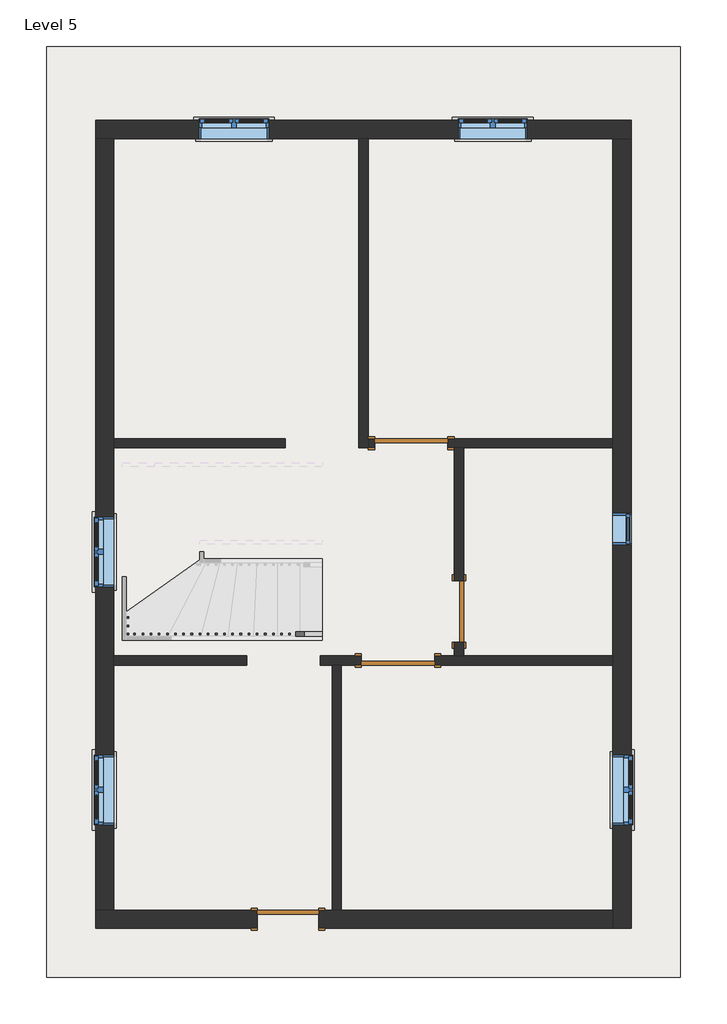
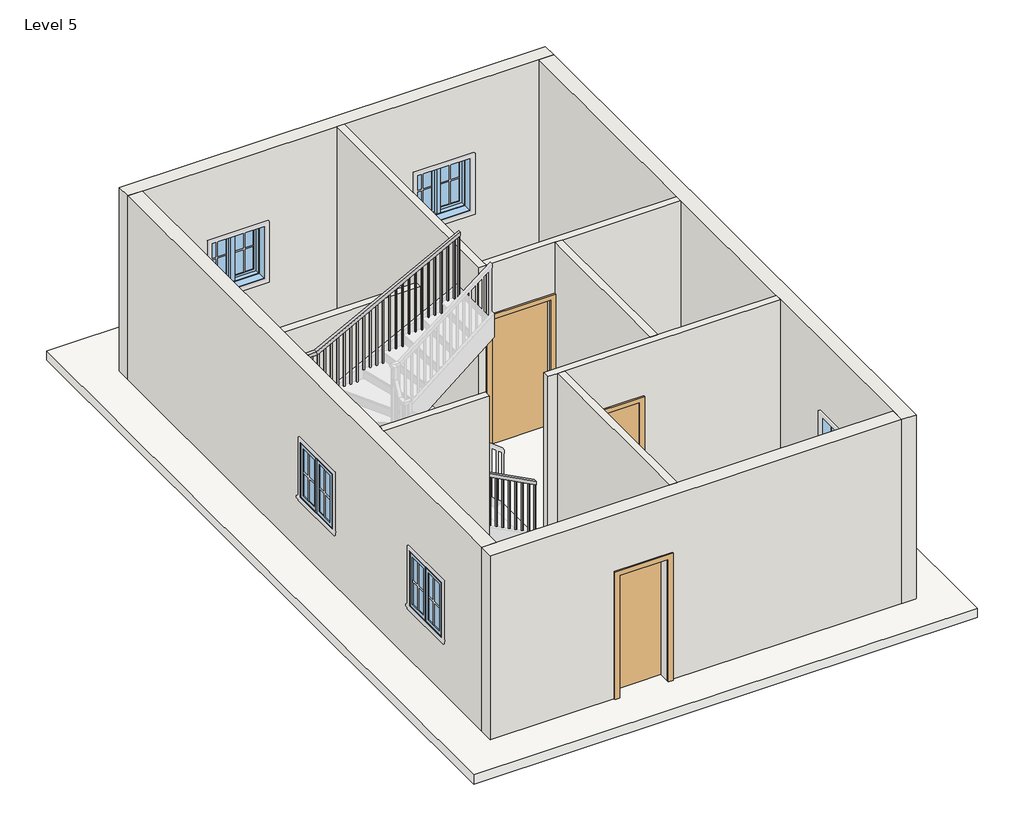
# One storey, part 1 of 2: 11 walls, 6 windows, 4 doors, 1 railing, 1 roof.
"""IFC4 building model written with IfcOpenShell, lengths in millimetres."""

from ifc_helpers import new_model, si_unit, frame, origin, place, context, project, spatial, polyline, outline, extrude, faceted_brep, transform, mapped, element, save
from components import door_d8f5dbb5, door_85036156, door_305aa2a5, door_e5f9f3c4, window_aa618e30, window_339605e1

model = new_model("IFC4")

# Units and contexts
model_context = context("Model", 3, world=origin())
ifc_project = project(units=[si_unit("LENGTHUNIT", "METRE", prefix="MILLI")], contexts=[model_context])

# Site, building, storey
site = spatial("IfcSite", under=ifc_project)
building = spatial("IfcBuilding", under=site)
storey = spatial("IfcBuildingStorey", under=building, Name="Level 5", Elevation=9601.2)

# Doors
placement = place(None, origin())
door_shape = door_d8f5dbb5(model_context)
element("IfcDoor", 1, ObjectType="Single-Flush : 30\" x 80\"", at=placement, inside=storey, context=model_context, shape_type="MappedRepresentation", body=[
    mapped(door_shape, transform((-82.2715692, -955.3070853, 9601.2), x_axis=(0.0, -1.0, 0.0), y_axis=(1.0, 0.0, 0.0), z_axis=(0.0, 0.0, 1.0))),
])
door_2_shape = door_85036156(model_context)
element("IfcDoor", 2, ObjectType="Single-Flush : 30\" x 80\"", at=placement, inside=storey, context=model_context, shape_type="MappedRepresentation", body=[
    mapped(door_2_shape, transform((-2212.5949167, -4784.3570853, 9601.2), x_axis=(-1.0, 0.0, 0.0), y_axis=(0.0, -1.0, 0.0), z_axis=(0.0, 0.0, 1.0))),
])
door_3_shape = door_305aa2a5(model_context)
element("IfcDoor", 3, ObjectType="Single-Flush : 36\" x 84\"", at=placement, inside=storey, context=model_context, shape_type="MappedRepresentation", body=[
    mapped(door_3_shape, transform((-677.5332429, 1140.1929147, 9601.2), x_axis=(-1.0, 0.0, 0.0), y_axis=(0.0, -1.0, 0.0), z_axis=(0.0, 0.0, 1.0))),
])
door_4_shape = door_e5f9f3c4(model_context)
element("IfcDoor", 4, ObjectType="Single-Flush : 36\" x 84\"", at=placement, inside=storey, context=model_context, shape_type="MappedRepresentation", body=[
    mapped(door_4_shape, transform((-842.6332429, -1564.9070853, 9601.2), x_axis=(-1.0, 0.0, 0.0), y_axis=(0.0, -1.0, 0.0), z_axis=(0.0, 0.0, 1.0))),
])

# Railing
element("IfcRailing", 5, ObjectType="Handrail - Rectangular", at=placement, inside=storey, context=model_context, shape_type="SolidModel", body=[
    faceted_brep([(-1783.4132248, -1260.1070853, 10684.9333333), (-1783.4132248, -1260.1070853, 10627.4742652), (-1783.4132248, -1209.3070853, 10627.4742652), (-1783.4132248, -1209.3070853, 10684.9333333), (-4041.1382869, -1260.1070853, 11878.2239201), (-4053.7373514, -1260.1070853, 11827.4239201), (-4053.7373514, -1209.3070853, 11827.4239201), (-4041.1382869, -1209.3070853, 11878.2239201), (-4225.5449167, -1260.1070853, 11878.2239201), (-4225.5449167, -1260.1070853, 11827.4239201), (-4174.7449167, -1209.3070853, 11827.4239201), (-4174.7449167, -1209.3070853, 11878.2239201), (-4225.5449167, -972.7952032, 11878.2239201), (-4225.5449167, -964.8446271, 11827.4239201), (-4174.7449167, -964.8446271, 11827.4239201), (-4174.7449167, -972.7952032, 11878.2239201), (-4225.5449167, 560.7810325, 12370.3094132), (-4225.5449167, 568.7316087, 12319.5094132), (-4174.7449167, 568.7316087, 12319.5094132), (-4174.7449167, 560.7810325, 12370.3094132), (-4225.5449167, 848.0929147, 12370.3094132), (-4225.5449167, 848.0929147, 12319.5094132), (-4174.7449167, 797.2929147, 12319.5094132), (-4174.7449167, 797.2929147, 12370.3094132), (-4041.1382869, 848.0929147, 12370.3094132), (-4028.5392223, 848.0929147, 12319.5094132), (-4028.5392223, 797.2929147, 12319.5094132), (-4041.1382869, 797.2929147, 12370.3094132), (-1783.4132248, 848.0929147, 13563.6), (-1783.4132248, 797.2929147, 13563.6), (-1783.4132248, 797.2929147, 13506.1409318), (-1783.4132248, 848.0929147, 13506.1409318)], [[[0, 1, 2, 3]], [[1, 0, 4, 5]], [[2, 1, 5, 6]], [[3, 2, 6, 7]], [[0, 3, 7, 4]], [[5, 4, 8, 9]], [[6, 5, 9, 10]], [[7, 6, 10, 11]], [[4, 7, 11, 8]], [[9, 8, 12, 13]], [[10, 9, 13, 14]], [[11, 10, 14, 15]], [[8, 11, 15, 12]], [[13, 12, 16, 17]], [[14, 13, 17, 18]], [[15, 14, 18, 19]], [[12, 15, 19, 16]], [[17, 16, 20, 21]], [[18, 17, 21, 22]], [[19, 18, 22, 23]], [[16, 19, 23, 20]], [[21, 20, 24, 25]], [[22, 21, 25, 26]], [[23, 22, 26, 27]], [[20, 23, 27, 24]], [[28, 29, 30, 31]], [[25, 24, 28, 31]], [[26, 25, 31, 30]], [[27, 26, 30, 29]], [[24, 27, 29, 28]]]),
    extrude(outline(polyline([(13458.8597858, -1872.8699167), (12479.8666667, -1872.8699167), (12479.8666667, -1853.8199167), (13468.9284102, -1853.8199167), (13458.8597858, -1872.8699167)])), frame((0.0, 813.1679147, 0.0), z_axis=(0.0, 1.0, 0.0), x_axis=(0.0, 0.0, 1.0)), (0.0, 0.0, 1.0), 19.05),
    extrude(outline(polyline([(13405.1604556, -1974.4699167), (12479.8666667, -1974.4699167), (12479.8666667, -1955.4199167), (13415.22908, -1955.4199167), (13405.1604556, -1974.4699167)])), frame((0.0, 813.1679147, 0.0), z_axis=(0.0, 1.0, 0.0), x_axis=(0.0, 0.0, 1.0)), (0.0, 0.0, 1.0), 19.05),
    extrude(outline(polyline([(13351.4611254, -2076.0699167), (12310.5333333, -2076.0699167), (12310.5333333, -2057.0199167), (13361.5297498, -2057.0199167), (13351.4611254, -2076.0699167)])), frame((0.0, 813.1679147, 0.0), z_axis=(0.0, 1.0, 0.0), x_axis=(0.0, 0.0, 1.0)), (0.0, 0.0, 1.0), 19.05),
    extrude(outline(polyline([(13297.7617952, -2177.6699167), (12310.5333333, -2177.6699167), (12310.5333333, -2158.6199167), (13307.8304196, -2158.6199167), (13297.7617952, -2177.6699167)])), frame((0.0, 813.1679147, 0.0), z_axis=(0.0, 1.0, 0.0), x_axis=(0.0, 0.0, 1.0)), (0.0, 0.0, 1.0), 19.05),
    extrude(outline(polyline([(13244.062465, -2279.2699167), (12310.5333333, -2279.2699167), (12310.5333333, -2260.2199167), (13254.1310894, -2260.2199167), (13244.062465, -2279.2699167)])), frame((0.0, 813.1679147, 0.0), z_axis=(0.0, 1.0, 0.0), x_axis=(0.0, 0.0, 1.0)), (0.0, 0.0, 1.0), 19.05),
    extrude(outline(polyline([(13190.3631348, -2380.8699167), (12141.2, -2380.8699167), (12141.2, -2361.8199167), (13200.4317592, -2361.8199167), (13190.3631348, -2380.8699167)])), frame((0.0, 813.1679147, 0.0), z_axis=(0.0, 1.0, 0.0), x_axis=(0.0, 0.0, 1.0)), (0.0, 0.0, 1.0), 19.05),
    extrude(outline(polyline([(13136.6638046, -2482.4699167), (12141.2, -2482.4699167), (12141.2, -2463.4199167), (13146.732429, -2463.4199167), (13136.6638046, -2482.4699167)])), frame((0.0, 813.1679147, 0.0), z_axis=(0.0, 1.0, 0.0), x_axis=(0.0, 0.0, 1.0)), (0.0, 0.0, 1.0), 19.05),
    extrude(outline(polyline([(13082.9644744, -2584.0699167), (12141.2, -2584.0699167), (12141.2, -2565.0199167), (13093.0330988, -2565.0199167), (13082.9644744, -2584.0699167)])), frame((0.0, 813.1679147, 0.0), z_axis=(0.0, 1.0, 0.0), x_axis=(0.0, 0.0, 1.0)), (0.0, 0.0, 1.0), 19.05),
    extrude(outline(polyline([(13029.2651442, -2685.6699167), (11971.8666667, -2685.6699167), (11971.8666667, -2666.6199167), (13039.3337686, -2666.6199167), (13029.2651442, -2685.6699167)])), frame((0.0, 813.1679147, 0.0), z_axis=(0.0, 1.0, 0.0), x_axis=(0.0, 0.0, 1.0)), (0.0, 0.0, 1.0), 19.05),
    extrude(outline(polyline([(12975.565814, -2787.2699167), (11971.8666667, -2787.2699167), (11971.8666667, -2768.2199167), (12985.6344384, -2768.2199167), (12975.565814, -2787.2699167)])), frame((0.0, 813.1679147, 0.0), z_axis=(0.0, 1.0, 0.0), x_axis=(0.0, 0.0, 1.0)), (0.0, 0.0, 1.0), 19.05),
    extrude(outline(polyline([(12921.8664838, -2888.8699167), (11971.8666667, -2888.8699167), (11971.8666667, -2869.8199167), (12931.9351082, -2869.8199167), (12921.8664838, -2888.8699167)])), frame((0.0, 813.1679147, 0.0), z_axis=(0.0, 1.0, 0.0), x_axis=(0.0, 0.0, 1.0)), (0.0, 0.0, 1.0), 19.05),
    extrude(outline(polyline([(12868.1671536, -2990.4699167), (11802.5333333, -2990.4699167), (11802.5333333, -2971.4199167), (12878.235778, -2971.4199167), (12868.1671536, -2990.4699167)])), frame((0.0, 813.1679147, 0.0), z_axis=(0.0, 1.0, 0.0), x_axis=(0.0, 0.0, 1.0)), (0.0, 0.0, 1.0), 19.05),
    extrude(outline(polyline([(12814.4678234, -3092.0699167), (11802.5333333, -3092.0699167), (11802.5333333, -3073.0199167), (12824.5364478, -3073.0199167), (12814.4678234, -3092.0699167)])), frame((0.0, 813.1679147, 0.0), z_axis=(0.0, 1.0, 0.0), x_axis=(0.0, 0.0, 1.0)), (0.0, 0.0, 1.0), 19.05),
    extrude(outline(polyline([(12760.7684932, -3193.6699167), (11802.5333333, -3193.6699167), (11802.5333333, -3174.6199167), (12770.8371176, -3174.6199167), (12760.7684932, -3193.6699167)])), frame((0.0, 813.1679147, 0.0), z_axis=(0.0, 1.0, 0.0), x_axis=(0.0, 0.0, 1.0)), (0.0, 0.0, 1.0), 19.05),
    extrude(outline(polyline([(12707.069163, -3295.2699167), (11802.5333333, -3295.2699167), (11802.5333333, -3276.2199167), (12717.1377874, -3276.2199167), (12707.069163, -3295.2699167)])), frame((0.0, 813.1679147, 0.0), z_axis=(0.0, 1.0, 0.0), x_axis=(0.0, 0.0, 1.0)), (0.0, 0.0, 1.0), 19.05),
    extrude(outline(polyline([(12653.3698328, -3396.8699167), (11633.2, -3396.8699167), (11633.2, -3377.8199167), (12663.4384572, -3377.8199167), (12653.3698328, -3396.8699167)])), frame((0.0, 813.1679147, 0.0), z_axis=(0.0, 1.0, 0.0), x_axis=(0.0, 0.0, 1.0)), (0.0, 0.0, 1.0), 19.05),
    extrude(outline(polyline([(12599.6705026, -3498.4699167), (11633.2, -3498.4699167), (11633.2, -3479.4199167), (12609.739127, -3479.4199167), (12599.6705026, -3498.4699167)])), frame((0.0, 813.1679147, 0.0), z_axis=(0.0, 1.0, 0.0), x_axis=(0.0, 0.0, 1.0)), (0.0, 0.0, 1.0), 19.05),
    extrude(outline(polyline([(12545.9711724, -3600.0699167), (11633.2, -3600.0699167), (11633.2, -3581.0199167), (12556.0397968, -3581.0199167), (12545.9711724, -3600.0699167)])), frame((0.0, 813.1679147, 0.0), z_axis=(0.0, 1.0, 0.0), x_axis=(0.0, 0.0, 1.0)), (0.0, 0.0, 1.0), 19.05),
    extrude(outline(polyline([(12492.2718422, -3701.6699167), (11633.2, -3701.6699167), (11633.2, -3682.6199167), (12502.3404666, -3682.6199167), (12492.2718422, -3701.6699167)])), frame((0.0, 813.1679147, 0.0), z_axis=(0.0, 1.0, 0.0), x_axis=(0.0, 0.0, 1.0)), (0.0, 0.0, 1.0), 19.05),
    extrude(outline(polyline([(12438.572512, -3803.2699167), (11463.8666667, -3803.2699167), (11463.8666667, -3784.2199167), (12448.6411364, -3784.2199167), (12438.572512, -3803.2699167)])), frame((0.0, 813.1679147, 0.0), z_axis=(0.0, 1.0, 0.0), x_axis=(0.0, 0.0, 1.0)), (0.0, 0.0, 1.0), 19.05),
    extrude(outline(polyline([(12384.8731818, -3904.8699167), (11463.8666667, -3904.8699167), (11463.8666667, -3885.8199167), (12394.9418062, -3885.8199167), (12384.8731818, -3904.8699167)])), frame((0.0, 813.1679147, 0.0), z_axis=(0.0, 1.0, 0.0), x_axis=(0.0, 0.0, 1.0)), (0.0, 0.0, 1.0), 19.05),
    extrude(outline(polyline([(12331.1738516, -4006.4699167), (11463.8666667, -4006.4699167), (11463.8666667, -3987.4199167), (12341.242476, -3987.4199167), (12331.1738516, -4006.4699167)])), frame((0.0, 813.1679147, 0.0), z_axis=(0.0, 1.0, 0.0), x_axis=(0.0, 0.0, 1.0)), (0.0, 0.0, 1.0), 19.05),
    extrude(outline(polyline([(-4108.0699167, 832.2179147), (-4089.0199167, 832.2179147), (-4089.0199167, 813.1679147), (-4108.0699167, 813.1679147), (-4108.0699167, 832.2179147)])), frame((0.0, 0.0, 11463.8666667), z_axis=(0.0, 0.0, 1.0), x_axis=(1.0, 0.0, 0.0)), (0.0, 0.0, 1.0), 855.6427466),
    extrude(outline(polyline([(-4209.6699167, 787.7679147), (-4209.6699167, 806.8179147), (-4190.6199167, 806.8179147), (-4190.6199167, 787.7679147), (-4209.6699167, 787.7679147)])), frame((0.0, 0.0, 11463.8666667), z_axis=(0.0, 0.0, 1.0), x_axis=(1.0, 0.0, 0.0)), (0.0, 0.0, 1.0), 855.6427466),
    extrude(outline(polyline([(-4209.6699167, 686.1679147), (-4209.6699167, 705.2179147), (-4190.6199167, 705.2179147), (-4190.6199167, 686.1679147), (-4209.6699167, 686.1679147)])), frame((0.0, 0.0, 11463.8666667), z_axis=(0.0, 0.0, 1.0), x_axis=(1.0, 0.0, 0.0)), (0.0, 0.0, 1.0), 855.6427466),
    extrude(outline(polyline([(-4209.6699167, 584.5679147), (-4209.6699167, 603.6179147), (-4190.6199167, 603.6179147), (-4190.6199167, 584.5679147), (-4209.6699167, 584.5679147)])), frame((0.0, 0.0, 11463.8666667), z_axis=(0.0, 0.0, 1.0), x_axis=(1.0, 0.0, 0.0)), (0.0, 0.0, 1.0), 855.6427466),
    extrude(outline(polyline([(502.0179147, 12298.1026907), (502.0179147, 11294.5333333), (482.9679147, 11294.5333333), (482.9679147, 12291.9900316), (502.0179147, 12298.1026907)])), frame((-4209.6699167, 0.0, 0.0), z_axis=(1.0, 0.0, 0.0), x_axis=(0.0, 1.0, 0.0)), (0.0, 0.0, 1.0), 19.05),
    extrude(outline(polyline([(400.4179147, 12265.5018425), (400.4179147, 11294.5333333), (381.3679147, 11294.5333333), (381.3679147, 12259.3891834), (400.4179147, 12265.5018425)])), frame((-4209.6699167, 0.0, 0.0), z_axis=(1.0, 0.0, 0.0), x_axis=(0.0, 1.0, 0.0)), (0.0, 0.0, 1.0), 19.05),
    extrude(outline(polyline([(298.8179147, 12232.9009942), (298.8179147, 11294.5333333), (279.7679147, 11294.5333333), (279.7679147, 12226.7883352), (298.8179147, 12232.9009942)])), frame((-4209.6699167, 0.0, 0.0), z_axis=(1.0, 0.0, 0.0), x_axis=(0.0, 1.0, 0.0)), (0.0, 0.0, 1.0), 19.05),
    extrude(outline(polyline([(197.2179147, 12200.300146), (197.2179147, 11294.5333333), (178.1679147, 11294.5333333), (178.1679147, 12194.187487), (197.2179147, 12200.300146)])), frame((-4209.6699167, 0.0, 0.0), z_axis=(1.0, 0.0, 0.0), x_axis=(0.0, 1.0, 0.0)), (0.0, 0.0, 1.0), 19.05),
    extrude(outline(polyline([(95.6179147, 12167.6992978), (95.6179147, 11294.5333333), (76.5679147, 11294.5333333), (76.5679147, 12161.5866387), (95.6179147, 12167.6992978)])), frame((-4209.6699167, 0.0, 0.0), z_axis=(1.0, 0.0, 0.0), x_axis=(0.0, 1.0, 0.0)), (0.0, 0.0, 1.0), 19.05),
    extrude(outline(polyline([(-5.9820853, 12135.0984495), (-5.9820853, 11125.2), (-25.0320853, 11125.2), (-25.0320853, 12128.9857905), (-5.9820853, 12135.0984495)])), frame((-4209.6699167, 0.0, 0.0), z_axis=(1.0, 0.0, 0.0), x_axis=(0.0, 1.0, 0.0)), (0.0, 0.0, 1.0), 19.05),
    extrude(outline(polyline([(-107.5820853, 12102.4976013), (-107.5820853, 11125.2), (-126.6320853, 11125.2), (-126.6320853, 12096.3849423), (-107.5820853, 12102.4976013)])), frame((-4209.6699167, 0.0, 0.0), z_axis=(1.0, 0.0, 0.0), x_axis=(0.0, 1.0, 0.0)), (0.0, 0.0, 1.0), 19.05),
    extrude(outline(polyline([(-209.1820853, 12069.8967531), (-209.1820853, 11125.2), (-228.2320853, 11125.2), (-228.2320853, 12063.784094), (-209.1820853, 12069.8967531)])), frame((-4209.6699167, 0.0, 0.0), z_axis=(1.0, 0.0, 0.0), x_axis=(0.0, 1.0, 0.0)), (0.0, 0.0, 1.0), 19.05),
    extrude(outline(polyline([(-310.7820853, 12037.2959049), (-310.7820853, 11125.2), (-329.8320853, 11125.2), (-329.8320853, 12031.1832458), (-310.7820853, 12037.2959049)])), frame((-4209.6699167, 0.0, 0.0), z_axis=(1.0, 0.0, 0.0), x_axis=(0.0, 1.0, 0.0)), (0.0, 0.0, 1.0), 19.05),
    extrude(outline(polyline([(-412.3820853, 12004.6950566), (-412.3820853, 11125.2), (-431.4320853, 11125.2), (-431.4320853, 11998.5823976), (-412.3820853, 12004.6950566)])), frame((-4209.6699167, 0.0, 0.0), z_axis=(1.0, 0.0, 0.0), x_axis=(0.0, 1.0, 0.0)), (0.0, 0.0, 1.0), 19.05),
    extrude(outline(polyline([(-513.9820853, 11972.0942084), (-513.9820853, 10955.8666667), (-533.0320853, 10955.8666667), (-533.0320853, 11965.9815494), (-513.9820853, 11972.0942084)])), frame((-4209.6699167, 0.0, 0.0), z_axis=(1.0, 0.0, 0.0), x_axis=(0.0, 1.0, 0.0)), (0.0, 0.0, 1.0), 19.05),
    extrude(outline(polyline([(-615.5820853, 11939.4933602), (-615.5820853, 10955.8666667), (-634.6320853, 10955.8666667), (-634.6320853, 11933.3807011), (-615.5820853, 11939.4933602)])), frame((-4209.6699167, 0.0, 0.0), z_axis=(1.0, 0.0, 0.0), x_axis=(0.0, 1.0, 0.0)), (0.0, 0.0, 1.0), 19.05),
    extrude(outline(polyline([(-717.1820853, 11906.892512), (-717.1820853, 10955.8666667), (-736.2320853, 10955.8666667), (-736.2320853, 11900.7798529), (-717.1820853, 11906.892512)])), frame((-4209.6699167, 0.0, 0.0), z_axis=(1.0, 0.0, 0.0), x_axis=(0.0, 1.0, 0.0)), (0.0, 0.0, 1.0), 19.05),
    extrude(outline(polyline([(-818.7820853, 11874.2916637), (-818.7820853, 10955.8666667), (-837.8320853, 10955.8666667), (-837.8320853, 11868.1790047), (-818.7820853, 11874.2916637)])), frame((-4209.6699167, 0.0, 0.0), z_axis=(1.0, 0.0, 0.0), x_axis=(0.0, 1.0, 0.0)), (0.0, 0.0, 1.0), 19.05),
    extrude(outline(polyline([(-920.3820853, 11841.6908155), (-920.3820853, 10955.8666667), (-939.4320853, 10955.8666667), (-939.4320853, 11835.5781565), (-920.3820853, 11841.6908155)])), frame((-4209.6699167, 0.0, 0.0), z_axis=(1.0, 0.0, 0.0), x_axis=(0.0, 1.0, 0.0)), (0.0, 0.0, 1.0), 19.05),
    extrude(outline(polyline([(-4209.6699167, -1041.0320853), (-4209.6699167, -1021.9820853), (-4190.6199167, -1021.9820853), (-4190.6199167, -1041.0320853), (-4209.6699167, -1041.0320853)])), frame((0.0, 0.0, 10786.5333333), z_axis=(0.0, 0.0, 1.0), x_axis=(1.0, 0.0, 0.0)), (0.0, 0.0, 1.0), 1040.8905868),
    extrude(outline(polyline([(-4209.6699167, -1142.6320853), (-4209.6699167, -1123.5820853), (-4190.6199167, -1123.5820853), (-4190.6199167, -1142.6320853), (-4209.6699167, -1142.6320853)])), frame((0.0, 0.0, 10786.5333333), z_axis=(0.0, 0.0, 1.0), x_axis=(1.0, 0.0, 0.0)), (0.0, 0.0, 1.0), 1040.8905868),
    extrude(outline(polyline([(-4110.6882248, -1244.2320853), (-4129.7382248, -1244.2320853), (-4129.7382248, -1225.1820853), (-4110.6882248, -1225.1820853), (-4110.6882248, -1244.2320853)])), frame((0.0, 0.0, 10786.5333333), z_axis=(0.0, 0.0, 1.0), x_axis=(1.0, 0.0, 0.0)), (0.0, 0.0, 1.0), 1040.8905868),
    extrude(outline(polyline([(11813.8938418, -4028.1382248), (10786.5333333, -4028.1382248), (10786.5333333, -4009.0882248), (11803.8252174, -4009.0882248), (11813.8938418, -4028.1382248)])), frame((0.0, -1244.2320853, 0.0), z_axis=(0.0, 1.0, 0.0), x_axis=(0.0, 0.0, 1.0)), (0.0, 0.0, 1.0), 19.05),
    extrude(outline(polyline([(11760.1945116, -3926.5382248), (10786.5333333, -3926.5382248), (10786.5333333, -3907.4882248), (11750.1258872, -3907.4882248), (11760.1945116, -3926.5382248)])), frame((0.0, -1244.2320853, 0.0), z_axis=(0.0, 1.0, 0.0), x_axis=(0.0, 0.0, 1.0)), (0.0, 0.0, 1.0), 19.05),
    extrude(outline(polyline([(11706.4951814, -3824.9382248), (10786.5333333, -3824.9382248), (10786.5333333, -3805.8882248), (11696.426557, -3805.8882248), (11706.4951814, -3824.9382248)])), frame((0.0, -1244.2320853, 0.0), z_axis=(0.0, 1.0, 0.0), x_axis=(0.0, 0.0, 1.0)), (0.0, 0.0, 1.0), 19.05),
    extrude(outline(polyline([(11652.7958512, -3723.3382248), (10786.5333333, -3723.3382248), (10786.5333333, -3704.2882248), (11642.7272268, -3704.2882248), (11652.7958512, -3723.3382248)])), frame((0.0, -1244.2320853, 0.0), z_axis=(0.0, 1.0, 0.0), x_axis=(0.0, 0.0, 1.0)), (0.0, 0.0, 1.0), 19.05),
    extrude(outline(polyline([(11599.096521, -3621.7382248), (10617.2, -3621.7382248), (10617.2, -3602.6882248), (11589.0278966, -3602.6882248), (11599.096521, -3621.7382248)])), frame((0.0, -1244.2320853, 0.0), z_axis=(0.0, 1.0, 0.0), x_axis=(0.0, 0.0, 1.0)), (0.0, 0.0, 1.0), 19.05),
    extrude(outline(polyline([(11545.3971908, -3520.1382248), (10617.2, -3520.1382248), (10617.2, -3501.0882248), (11535.3285664, -3501.0882248), (11545.3971908, -3520.1382248)])), frame((0.0, -1244.2320853, 0.0), z_axis=(0.0, 1.0, 0.0), x_axis=(0.0, 0.0, 1.0)), (0.0, 0.0, 1.0), 19.05),
    extrude(outline(polyline([(11491.6978606, -3418.5382248), (10617.2, -3418.5382248), (10617.2, -3399.4882248), (11481.6292362, -3399.4882248), (11491.6978606, -3418.5382248)])), frame((0.0, -1244.2320853, 0.0), z_axis=(0.0, 1.0, 0.0), x_axis=(0.0, 0.0, 1.0)), (0.0, 0.0, 1.0), 19.05),
    extrude(outline(polyline([(11437.9985304, -3316.9382248), (10617.2, -3316.9382248), (10617.2, -3297.8882248), (11427.929906, -3297.8882248), (11437.9985304, -3316.9382248)])), frame((0.0, -1244.2320853, 0.0), z_axis=(0.0, 1.0, 0.0), x_axis=(0.0, 0.0, 1.0)), (0.0, 0.0, 1.0), 19.05),
    extrude(outline(polyline([(11384.2992002, -3215.3382248), (10447.8666667, -3215.3382248), (10447.8666667, -3196.2882248), (11374.2305758, -3196.2882248), (11384.2992002, -3215.3382248)])), frame((0.0, -1244.2320853, 0.0), z_axis=(0.0, 1.0, 0.0), x_axis=(0.0, 0.0, 1.0)), (0.0, 0.0, 1.0), 19.05),
    extrude(outline(polyline([(11330.59987, -3113.7382248), (10447.8666667, -3113.7382248), (10447.8666667, -3094.6882248), (11320.5312456, -3094.6882248), (11330.59987, -3113.7382248)])), frame((0.0, -1244.2320853, 0.0), z_axis=(0.0, 1.0, 0.0), x_axis=(0.0, 0.0, 1.0)), (0.0, 0.0, 1.0), 19.05),
    extrude(outline(polyline([(11276.9005398, -3012.1382248), (10447.8666667, -3012.1382248), (10447.8666667, -2993.0882248), (11266.8319154, -2993.0882248), (11276.9005398, -3012.1382248)])), frame((0.0, -1244.2320853, 0.0), z_axis=(0.0, 1.0, 0.0), x_axis=(0.0, 0.0, 1.0)), (0.0, 0.0, 1.0), 19.05),
    extrude(outline(polyline([(11223.2012096, -2910.5382248), (10278.5333333, -2910.5382248), (10278.5333333, -2891.4882248), (11213.1325852, -2891.4882248), (11223.2012096, -2910.5382248)])), frame((0.0, -1244.2320853, 0.0), z_axis=(0.0, 1.0, 0.0), x_axis=(0.0, 0.0, 1.0)), (0.0, 0.0, 1.0), 19.05),
    extrude(outline(polyline([(11169.5018794, -2808.9382248), (10278.5333333, -2808.9382248), (10278.5333333, -2789.8882248), (11159.433255, -2789.8882248), (11169.5018794, -2808.9382248)])), frame((0.0, -1244.2320853, 0.0), z_axis=(0.0, 1.0, 0.0), x_axis=(0.0, 0.0, 1.0)), (0.0, 0.0, 1.0), 19.05),
    extrude(outline(polyline([(11115.8025492, -2707.3382248), (10278.5333333, -2707.3382248), (10278.5333333, -2688.2882248), (11105.7339248, -2688.2882248), (11115.8025492, -2707.3382248)])), frame((0.0, -1244.2320853, 0.0), z_axis=(0.0, 1.0, 0.0), x_axis=(0.0, 0.0, 1.0)), (0.0, 0.0, 1.0), 19.05),
    extrude(outline(polyline([(11062.103219, -2605.7382248), (10109.2, -2605.7382248), (10109.2, -2586.6882248), (11052.0345946, -2586.6882248), (11062.103219, -2605.7382248)])), frame((0.0, -1244.2320853, 0.0), z_axis=(0.0, 1.0, 0.0), x_axis=(0.0, 0.0, 1.0)), (0.0, 0.0, 1.0), 19.05),
    extrude(outline(polyline([(11008.4038888, -2504.1382248), (10109.2, -2504.1382248), (10109.2, -2485.0882248), (10998.3352644, -2485.0882248), (11008.4038888, -2504.1382248)])), frame((0.0, -1244.2320853, 0.0), z_axis=(0.0, 1.0, 0.0), x_axis=(0.0, 0.0, 1.0)), (0.0, 0.0, 1.0), 19.05),
    extrude(outline(polyline([(10954.7045586, -2402.5382248), (10109.2, -2402.5382248), (10109.2, -2383.4882248), (10944.6359342, -2383.4882248), (10954.7045586, -2402.5382248)])), frame((0.0, -1244.2320853, 0.0), z_axis=(0.0, 1.0, 0.0), x_axis=(0.0, 0.0, 1.0)), (0.0, 0.0, 1.0), 19.05),
    extrude(outline(polyline([(10901.0052284, -2300.9382248), (9939.8666667, -2300.9382248), (9939.8666667, -2281.8882248), (10890.936604, -2281.8882248), (10901.0052284, -2300.9382248)])), frame((0.0, -1244.2320853, 0.0), z_axis=(0.0, 1.0, 0.0), x_axis=(0.0, 0.0, 1.0)), (0.0, 0.0, 1.0), 19.05),
    extrude(outline(polyline([(10847.3058982, -2199.3382248), (9939.8666667, -2199.3382248), (9939.8666667, -2180.2882248), (10837.2372738, -2180.2882248), (10847.3058982, -2199.3382248)])), frame((0.0, -1244.2320853, 0.0), z_axis=(0.0, 1.0, 0.0), x_axis=(0.0, 0.0, 1.0)), (0.0, 0.0, 1.0), 19.05),
    extrude(outline(polyline([(10793.606568, -2097.7382248), (9939.8666667, -2097.7382248), (9939.8666667, -2078.6882248), (10783.5379436, -2078.6882248), (10793.606568, -2097.7382248)])), frame((0.0, -1244.2320853, 0.0), z_axis=(0.0, 1.0, 0.0), x_axis=(0.0, 0.0, 1.0)), (0.0, 0.0, 1.0), 19.05),
    extrude(outline(polyline([(10739.9072378, -1996.1382248), (9770.5333333, -1996.1382248), (9770.5333333, -1977.0882248), (10729.8386134, -1977.0882248), (10739.9072378, -1996.1382248)])), frame((0.0, -1244.2320853, 0.0), z_axis=(0.0, 1.0, 0.0), x_axis=(0.0, 0.0, 1.0)), (0.0, 0.0, 1.0), 19.05),
    extrude(outline(polyline([(10686.2079076, -1894.5382248), (9770.5333333, -1894.5382248), (9770.5333333, -1875.4882248), (10676.1392831, -1875.4882248), (10686.2079076, -1894.5382248)])), frame((0.0, -1244.2320853, 0.0), z_axis=(0.0, 1.0, 0.0), x_axis=(0.0, 0.0, 1.0)), (0.0, 0.0, 1.0), 19.05),
    extrude(outline(polyline([(-4209.6699167, 813.1679147), (-4209.6699167, 832.2179147), (-4190.6199167, 832.2179147), (-4190.6199167, 813.1679147), (-4209.6699167, 813.1679147)])), frame((0.0, 0.0, 11463.8666667), z_axis=(0.0, 0.0, 1.0), x_axis=(1.0, 0.0, 0.0)), (0.0, 0.0, 1.0), 855.6427466),
    extrude(outline(polyline([(-4190.6199167, -1244.2320853), (-4209.6699167, -1244.2320853), (-4209.6699167, -1225.1820853), (-4190.6199167, -1225.1820853), (-4190.6199167, -1244.2320853)])), frame((0.0, 0.0, 10786.5333333), z_axis=(0.0, 0.0, 1.0), x_axis=(1.0, 0.0, 0.0)), (0.0, 0.0, 1.0), 1040.8905868),
    extrude(outline(polyline([(13496.0723074, -1802.4632248), (12479.8666667, -1802.4632248), (12479.8666667, -1783.4132248), (13506.1409318, -1783.4132248), (13496.0723074, -1802.4632248)])), frame((0.0, 813.1679147, 0.0), z_axis=(0.0, 1.0, 0.0), x_axis=(0.0, 0.0, 1.0)), (0.0, 0.0, 1.0), 19.05),
    extrude(outline(polyline([(10637.5428896, -1802.4632248), (9770.5333333, -1802.4632248), (9770.5333333, -1783.4132248), (10627.4742652, -1783.4132248), (10637.5428896, -1802.4632248)])), frame((0.0, -1244.2320853, 0.0), z_axis=(0.0, 1.0, 0.0), x_axis=(0.0, 0.0, 1.0)), (0.0, 0.0, 1.0), 19.05),
])

# Roof
element("IfcRoof", 6, ObjectType="Generic - 12\"", at=placement, inside=storey, context=model_context, shape_type="SweptSolid", body=[
    extrude(outline(polyline([(-5216.1449167, 6076.3773594), (2670.5550833, 6076.3773594), (2670.5550833, -5508.2570853), (-5216.1449167, -5508.2570853), (-5216.1449167, 6076.3773594)])), frame((0.0, 0.0, 9448.8), z_axis=(0.0, 0.0, 1.0), x_axis=(1.0, 0.0, 0.0)), (0.0, 0.0, 1.0), 152.4),
])

# Walls
element("IfcWall", 7, ObjectType="WALL4.5\"", at=placement, inside=storey, context=model_context, shape_type="Brep", body=[
    faceted_brep([(-1329.9449167, 4931.1429147, 9601.2), (-1329.9449167, 1083.0429147, 9601.2), (-1329.9449167, 1083.0429147, 12649.2), (-1329.9449167, 4931.1429147, 12649.2), (-1215.6449167, 4931.1429147, 9601.2), (-1215.6449167, 4931.1429147, 12649.2), (-1215.6449167, 1197.3429147, 12649.2), (-1215.6449167, 1083.0429147, 12649.2), (-1215.6449167, 1083.0429147, 9601.2), (-1215.6449167, 1197.3429147, 9601.2)], [[[0, 1, 2, 3]], [[4, 5, 6, 7, 8, 9]], [[1, 0, 4, 9, 8]], [[0, 3, 5, 4]], [[2, 1, 8, 7]], [[3, 2, 7, 6, 5]]]),
])
element("IfcWall", 8, ObjectType="WALL4.5\"", at=placement, inside=storey, context=model_context, shape_type="Brep", body=[
    faceted_brep([(-1215.6449167, 1083.0429147, 9601.2), (-1134.7332429, 1083.0429147, 9601.2), (-1134.7332429, 1083.0429147, 11734.8), (-220.3332429, 1083.0429147, 11734.8), (-220.3332429, 1083.0429147, 9601.2), (-139.4215692, 1083.0429147, 9601.2), (-25.1215692, 1083.0429147, 9601.2), (1832.3550833, 1083.0429147, 9601.2), (1832.3550833, 1083.0429147, 12649.2), (-25.1215692, 1083.0429147, 12649.2), (-139.4215692, 1083.0429147, 12649.2), (-1215.6449167, 1083.0429147, 12649.2), (-1134.7332429, 1197.3429147, 11734.8), (-1134.7332429, 1197.3429147, 9601.2), (-1215.6449167, 1197.3429147, 9601.2), (-1215.6449167, 1197.3429147, 12649.2), (1832.3550833, 1197.3429147, 12649.2), (1832.3550833, 1197.3429147, 9601.2), (-220.3332429, 1197.3429147, 9601.2), (-220.3332429, 1197.3429147, 11734.8)], [[[0, 1, 2, 3, 4, 5, 6, 7, 8, 9, 10, 11]], [[12, 13, 14, 15, 16, 17, 18, 19]], [[18, 17, 7, 6, 5, 4]], [[14, 13, 1, 0]], [[0, 11, 15, 14]], [[8, 7, 17, 16]], [[2, 1, 13, 12]], [[3, 2, 12, 19]], [[4, 3, 19, 18]], [[11, 10, 9, 8, 16, 15]]]),
])
element("IfcWall", 9, ObjectType="WALL4.5\"", at=placement, inside=storey, context=model_context, shape_type="SweptSolid", body=[
    extrude(outline(polyline([(-2244.3449167, 1083.0429147), (-4377.9449167, 1083.0429147), (-4377.9449167, 1197.3429147), (-2244.3449167, 1197.3429147), (-2244.3449167, 1083.0429147)])), frame((0.0, 0.0, 9601.2), z_axis=(0.0, 0.0, 1.0), x_axis=(1.0, 0.0, 0.0)), (0.0, 0.0, 1.0), 3048.0),
])
element("IfcWall", 10, ObjectType="WALL4.5\"", at=placement, inside=storey, context=model_context, shape_type="SweptSolid", body=[
    extrude(outline(polyline([(-1336.3070853, 11633.2), (-1336.3070853, 9601.2), (-1507.7570853, 9601.2), (-1507.7570853, 12649.2), (1083.0429147, 12649.2), (1083.0429147, 9601.2), (-574.3070853, 9601.2), (-574.3070853, 11633.2), (-1336.3070853, 11633.2)])), frame((-139.4215692, 0.0, 0.0), z_axis=(1.0, 0.0, 0.0), x_axis=(0.0, 1.0, 0.0)), (0.0, 0.0, 1.0), 114.3),
])
element("IfcWall", 11, ObjectType="WALL4.5\"", at=placement, inside=storey, context=model_context, shape_type="SweptSolid", body=[
    extrude(outline(polyline([(-2726.9449167, -1622.0570853), (-4377.9449167, -1622.0570853), (-4377.9449167, -1507.7570853), (-2726.9449167, -1507.7570853), (-2726.9449167, -1622.0570853)])), frame((0.0, 0.0, 9601.2), z_axis=(0.0, 0.0, 1.0), x_axis=(1.0, 0.0, 0.0)), (0.0, 0.0, 1.0), 3048.0),
])
element("IfcWall", 12, ObjectType="WALL4.5\"", at=placement, inside=storey, context=model_context, shape_type="Brep", body=[
    faceted_brep([(-1812.5449167, -1622.0570853, 9601.2), (-1660.1449167, -1622.0570853, 9601.2), (-1545.8449167, -1622.0570853, 9601.2), (-1299.8332429, -1622.0570853, 9601.2), (-1299.8332429, -1622.0570853, 11734.8), (-385.4332429, -1622.0570853, 11734.8), (-385.4332429, -1622.0570853, 9601.2), (1832.3550833, -1622.0570853, 9601.2), (1832.3550833, -1622.0570853, 12649.2), (-1545.8449167, -1622.0570853, 12649.2), (-1660.1449167, -1622.0570853, 12649.2), (-1812.5449167, -1622.0570853, 12649.2), (-1299.8332429, -1507.7570853, 11734.8), (-1299.8332429, -1507.7570853, 9601.2), (-1812.5449167, -1507.7570853, 9601.2), (-1812.5449167, -1507.7570853, 12649.2), (-139.4215692, -1507.7570853, 12649.2), (-25.1215692, -1507.7570853, 12649.2), (1832.3550833, -1507.7570853, 12649.2), (1832.3550833, -1507.7570853, 9601.2), (-25.1215692, -1507.7570853, 9601.2), (-139.4215692, -1507.7570853, 9601.2), (-385.4332429, -1507.7570853, 9601.2), (-385.4332429, -1507.7570853, 11734.8)], [[[0, 1, 2, 3, 4, 5, 6, 7, 8, 9, 10, 11]], [[12, 13, 14, 15, 16, 17, 18, 19, 20, 21, 22, 23]], [[14, 13, 3, 2, 1, 0]], [[22, 21, 20, 19, 7, 6]], [[0, 11, 15, 14]], [[8, 7, 19, 18]], [[4, 3, 13, 12]], [[5, 4, 12, 23]], [[6, 5, 23, 22]], [[11, 10, 9, 8, 18, 17, 16, 15]]]),
])
element("IfcWall", 13, ObjectType="WALL4.5\"", at=placement, inside=storey, context=model_context, shape_type="SweptSolid", body=[
    extrude(outline(polyline([(-1660.1449167, -4670.0570853), (-1660.1449167, -1622.0570853), (-1545.8449167, -1622.0570853), (-1545.8449167, -4670.0570853), (-1660.1449167, -4670.0570853)])), frame((0.0, 0.0, 9601.2), z_axis=(0.0, 0.0, 1.0), x_axis=(1.0, 0.0, 0.0)), (0.0, 0.0, 1.0), 3048.0),
])
element("IfcWall", 14, ObjectType="WALL9\"", at=placement, inside=storey, context=model_context, shape_type="Brep", body=[
    faceted_brep([(-4606.5449167, 4931.1429147, 9601.2), (-4377.9449167, 4931.1429147, 9601.2), (-1329.9449167, 4931.1429147, 9601.2), (-1215.6449167, 4931.1429147, 9601.2), (1832.3550833, 4931.1429147, 9601.2), (2060.9550833, 4931.1429147, 9601.2), (2060.9550833, 4931.1429147, 12649.2), (1832.3550833, 4931.1429147, 12649.2), (-1215.6449167, 4931.1429147, 12649.2), (-1329.9449167, 4931.1429147, 12649.2), (-4377.9449167, 4931.1429147, 12649.2), (-4606.5449167, 4931.1429147, 12649.2), (-2450.7199167, 4931.1429147, 11430.0), (-2450.7199167, 4931.1429147, 10515.6), (-3314.3199167, 4931.1429147, 10515.6), (-3314.3199167, 4931.1429147, 11430.0), (768.7300833, 4931.1429147, 11430.0), (768.7300833, 4931.1429147, 10515.6), (-94.8699167, 4931.1429147, 10515.6), (-94.8699167, 4931.1429147, 11430.0), (-4606.5449167, 5159.7429147, 9601.2), (-4606.5449167, 5159.7429147, 12649.2), (2060.9550833, 5159.7429147, 12649.2), (2060.9550833, 5159.7429147, 9601.2), (-2450.7199167, 5159.7429147, 11430.0), (-3314.3199167, 5159.7429147, 11430.0), (-3314.3199167, 5159.7429147, 10515.6), (-2450.7199167, 5159.7429147, 10515.6), (768.7300833, 5159.7429147, 11430.0), (-94.8699167, 5159.7429147, 11430.0), (-94.8699167, 5159.7429147, 10515.6), (768.7300833, 5159.7429147, 10515.6)], [[[0, 1, 2, 3, 4, 5, 6, 7, 8, 9, 10, 11], [12, 13, 14, 15], [16, 17, 18, 19]], [[20, 21, 22, 23], [24, 25, 26, 27], [28, 29, 30, 31]], [[5, 4, 3, 2, 1, 0, 20, 23]], [[6, 5, 23, 22]], [[0, 11, 21, 20]], [[13, 12, 24, 27]], [[14, 13, 27, 26]], [[15, 14, 26, 25]], [[12, 15, 25, 24]], [[17, 16, 28, 31]], [[18, 17, 31, 30]], [[19, 18, 30, 29]], [[16, 19, 29, 28]], [[11, 10, 9, 8, 7, 6, 22, 21]]]),
])
element("IfcWall", 15, ObjectType="WALL9\"", at=placement, inside=storey, context=model_context, shape_type="Brep", body=[
    faceted_brep([(1832.3550833, 4931.1429147, 9601.2), (1832.3550833, 1197.3429147, 9601.2), (1832.3550833, 1083.0429147, 9601.2), (1832.3550833, -1507.7570853, 9601.2), (1832.3550833, -1622.0570853, 9601.2), (1832.3550833, -4670.0570853, 9601.2), (1832.3550833, -4898.6570853, 9601.2), (1832.3550833, -4898.6570853, 12649.2), (1832.3550833, -4670.0570853, 12649.2), (1832.3550833, -1622.0570853, 12649.2), (1832.3550833, -1507.7570853, 12649.2), (1832.3550833, 1083.0429147, 12649.2), (1832.3550833, 1197.3429147, 12649.2), (1832.3550833, 4931.1429147, 12649.2), (1832.3550833, -129.8070853, 11125.2), (1832.3550833, -129.8070853, 10515.6), (1832.3550833, 276.5929147, 10515.6), (1832.3550833, 276.5929147, 11125.2), (1832.3550833, -3606.4320853, 11430.0), (1832.3550833, -3606.4320853, 10515.6), (1832.3550833, -2742.8320853, 10515.6), (1832.3550833, -2742.8320853, 11430.0), (2060.9550833, 4931.1429147, 9601.2), (2060.9550833, 4931.1429147, 12649.2), (2060.9550833, -4898.6570853, 12649.2), (2060.9550833, -4898.6570853, 9601.2), (2060.9550833, -129.8070853, 11125.2), (2060.9550833, 276.5929147, 11125.2), (2060.9550833, 276.5929147, 10515.6), (2060.9550833, -129.8070853, 10515.6), (2060.9550833, -3606.4320853, 11430.0), (2060.9550833, -2742.8320853, 11430.0), (2060.9550833, -2742.8320853, 10515.6), (2060.9550833, -3606.4320853, 10515.6)], [[[0, 1, 2, 3, 4, 5, 6, 7, 8, 9, 10, 11, 12, 13], [14, 15, 16, 17], [18, 19, 20, 21]], [[22, 23, 24, 25], [26, 27, 28, 29], [30, 31, 32, 33]], [[6, 5, 4, 3, 2, 1, 0, 22, 25]], [[0, 13, 23, 22]], [[7, 6, 25, 24]], [[15, 14, 26, 29]], [[16, 15, 29, 28]], [[17, 16, 28, 27]], [[14, 17, 27, 26]], [[19, 18, 30, 33]], [[20, 19, 33, 32]], [[21, 20, 32, 31]], [[18, 21, 31, 30]], [[13, 12, 11, 10, 9, 8, 7, 24, 23]]]),
])
element("IfcWall", 16, ObjectType="WALL9\"", at=placement, inside=storey, context=model_context, shape_type="Brep", body=[
    faceted_brep([(-2593.5949167, -4670.0570853, 11633.2), (-2593.5949167, -4670.0570853, 9601.2), (-4377.9449167, -4670.0570853, 9601.2), (-4606.5449167, -4670.0570853, 9601.2), (-4606.5449167, -4670.0570853, 12649.2), (-4377.9449167, -4670.0570853, 12649.2), (-1660.1449167, -4670.0570853, 12649.2), (-1545.8449167, -4670.0570853, 12649.2), (1832.3550833, -4670.0570853, 12649.2), (1832.3550833, -4670.0570853, 9601.2), (-1545.8449167, -4670.0570853, 9601.2), (-1660.1449167, -4670.0570853, 9601.2), (-1831.5949167, -4670.0570853, 9601.2), (-1831.5949167, -4670.0570853, 11633.2), (-4606.5449167, -4898.6570853, 9601.2), (-2593.5949167, -4898.6570853, 9601.2), (-2593.5949167, -4898.6570853, 11633.2), (-1831.5949167, -4898.6570853, 11633.2), (-1831.5949167, -4898.6570853, 9601.2), (1832.3550833, -4898.6570853, 9601.2), (1832.3550833, -4898.6570853, 12649.2), (-4606.5449167, -4898.6570853, 12649.2)], [[[0, 1, 2, 3, 4, 5, 6, 7, 8, 9, 10, 11, 12, 13]], [[14, 15, 16, 17, 18, 19, 20, 21]], [[3, 2, 1, 15, 14]], [[12, 11, 10, 9, 19, 18]], [[9, 8, 20, 19]], [[4, 3, 14, 21]], [[16, 15, 1, 0]], [[17, 16, 0, 13]], [[18, 17, 13, 12]], [[8, 7, 6, 5, 4, 21, 20]]]),
])
element("IfcWall", 17, ObjectType="WALL9\"", at=placement, inside=storey, context=model_context, shape_type="Brep", body=[
    faceted_brep([(-4377.9449167, -4670.0570853, 9601.2), (-4377.9449167, -1622.0570853, 9601.2), (-4377.9449167, -1507.7570853, 9601.2), (-4377.9449167, 1083.0429147, 9601.2), (-4377.9449167, 1197.3429147, 9601.2), (-4377.9449167, 4931.1429147, 9601.2), (-4377.9449167, 4931.1429147, 12649.2), (-4377.9449167, 1197.3429147, 12649.2), (-4377.9449167, 1083.0429147, 12649.2), (-4377.9449167, -1507.7570853, 12649.2), (-4377.9449167, -1622.0570853, 12649.2), (-4377.9449167, -4670.0570853, 12649.2), (-4377.9449167, -2742.8320853, 11430.0), (-4377.9449167, -2742.8320853, 10515.6), (-4377.9449167, -3606.4320853, 10515.6), (-4377.9449167, -3606.4320853, 11430.0), (-4377.9449167, 219.4429147, 11430.0), (-4377.9449167, 219.4429147, 10515.6), (-4377.9449167, -644.1570853, 10515.6), (-4377.9449167, -644.1570853, 11430.0), (-4606.5449167, -4670.0570853, 9601.2), (-4606.5449167, -4670.0570853, 12649.2), (-4606.5449167, 4931.1429147, 12649.2), (-4606.5449167, 4931.1429147, 9601.2), (-4606.5449167, -2742.8320853, 11430.0), (-4606.5449167, -3606.4320853, 11430.0), (-4606.5449167, -3606.4320853, 10515.6), (-4606.5449167, -2742.8320853, 10515.6), (-4606.5449167, 219.4429147, 11430.0), (-4606.5449167, -644.1570853, 11430.0), (-4606.5449167, -644.1570853, 10515.6), (-4606.5449167, 219.4429147, 10515.6)], [[[0, 1, 2, 3, 4, 5, 6, 7, 8, 9, 10, 11], [12, 13, 14, 15], [16, 17, 18, 19]], [[20, 21, 22, 23], [24, 25, 26, 27], [28, 29, 30, 31]], [[5, 4, 3, 2, 1, 0, 20, 23]], [[0, 11, 21, 20]], [[6, 5, 23, 22]], [[13, 12, 24, 27]], [[14, 13, 27, 26]], [[15, 14, 26, 25]], [[12, 15, 25, 24]], [[17, 16, 28, 31]], [[18, 17, 31, 30]], [[19, 18, 30, 29]], [[16, 19, 29, 28]], [[11, 10, 9, 8, 7, 6, 22, 21]]]),
])

# Windows
window_shape = window_aa618e30(model_context)
element("IfcWindow", 18, ObjectType="Fixed : 16\" x 24\"", at=placement, inside=storey, context=model_context, shape_type="MappedRepresentation", body=[
    mapped(window_shape, transform((1946.6550833, 35.2929147, 9601.2), x_axis=(0.0, -1.0, 0.0), y_axis=(1.0, 0.0, 0.0), z_axis=(0.0, 0.0, 1.0))),
])
window_2_shape = window_339605e1(model_context)
element("IfcWindow", 19, ObjectType="Window-Casement-Double : 34\" x 36\"", at=placement, inside=storey, context=model_context, shape_type="MappedRepresentation", body=[
    mapped(window_2_shape, transform((-2882.5199167, 5045.4429147, 9601.2), x_axis=(1.0, 0.0, 0.0), y_axis=(0.0, 1.0, 0.0), z_axis=(0.0, 0.0, 1.0))),
])
element("IfcWindow", 20, ObjectType="Window-Casement-Double : 34\" x 36\"", at=placement, inside=storey, context=model_context, shape_type="MappedRepresentation", body=[
    mapped(window_2_shape, transform((336.9300833, 5045.4429147, 9601.2), x_axis=(1.0, 0.0, 0.0), y_axis=(0.0, 1.0, 0.0), z_axis=(0.0, 0.0, 1.0))),
])
element("IfcWindow", 21, ObjectType="Window-Casement-Double : 34\" x 36\"", at=placement, inside=storey, context=model_context, shape_type="MappedRepresentation", body=[
    mapped(window_2_shape, transform((1946.6550833, -3174.6320853, 9601.2), x_axis=(0.0, -1.0, 0.0), y_axis=(1.0, 0.0, 0.0), z_axis=(0.0, 0.0, 1.0))),
])
element("IfcWindow", 22, ObjectType="Window-Casement-Double : 34\" x 36\"", at=placement, inside=storey, context=model_context, shape_type="MappedRepresentation", body=[
    mapped(window_2_shape, transform((-4492.2449167, -3174.6320853, 9601.2), x_axis=(0.0, 1.0, 0.0), y_axis=(-1.0, 0.0, 0.0), z_axis=(0.0, 0.0, 1.0))),
])
element("IfcWindow", 23, ObjectType="Window-Casement-Double : 34\" x 36\"", at=placement, inside=storey, context=model_context, shape_type="MappedRepresentation", body=[
    mapped(window_2_shape, transform((-4492.2449167, -212.3570853, 9601.2), x_axis=(0.0, 1.0, 0.0), y_axis=(-1.0, 0.0, 0.0), z_axis=(0.0, 0.0, 1.0))),
])

save(model, "model.ifc")

# Revit data of these elements
# Type "Single-Flush : 30\" x 80\""
#   Type Mark = "5"
#   Construction Type Id = "MDOOR"
#   Assembly Code = "C1020"
#   Analytic Construction = "Metal"
#   Thickness = 0' - 2"
#   Heat Transfer Coefficient (U) = 0.651978 BTU/(h·ft²·°F)
#   Height = 6' - 8"
#   Trim Projection Ext = 0' - 1"
#   Trim Projection Int = 0' - 1"
#   Trim Width = 0' - 3"
#   Width = 2' - 6"
#   Define Thermal Properties by = 1
#   Define Thermal Properties by = 1
#   Door Material = Door - Panel
#   Frame Material = Door - Frame
#   Visual Light Transmittance = 0
#   Solar Heat Gain Coefficient = 0
#   Function = (empty or 0)
#   Wall Closure = (empty or 0)
# Type "Single-Flush : 36\" x 84\""
#   Type Mark = "1"
#   Construction Type Id = "MDOOR"
#   Assembly Code = "C1020"
#   Analytic Construction = "Metal"
#   Thickness = 0' - 2"
#   Heat Transfer Coefficient (U) = 0.651978 BTU/(h·ft²·°F)
#   Height = 7' - 0"
#   Trim Projection Ext = 0' - 1"
#   Trim Projection Int = 0' - 1"
#   Trim Width = 0' - 3"
#   Width = 3' - 0"
#   Define Thermal Properties by = 1
#   Define Thermal Properties by = 1
#   Door Material = Door - Panel
#   Frame Material = Door - Frame
#   Visual Light Transmittance = 0
#   Solar Heat Gain Coefficient = 0
#   Function = (empty or 0)
#   Wall Closure = (empty or 0)
# Type "Handrail - Rectangular"
#   Assembly Code = "C2010400"
#   built-in parameter 1008612 = 0.0416667 (stored number, unit not read)
#   built-in parameter 1008611 = 0.0416667 (stored number, unit not read)
#   built-in parameter 1008609 = 0.333333 (stored number, unit not read)
#   built-in parameter 1008604 = 0.166667 (stored number, unit not read)
#   built-in parameter 1008603 = 0.166667 (stored number, unit not read)
#   Railing Height = 3' - 0"
#   built-in parameter 1008630 = 2
#   built-in parameter 1008610 = 2
#   built-in parameter 1008618 = Baluster - Square : 3/4"
# Type "Generic - 12\""
#   Assembly Code = "B1020"
#   Layers, outside or top first: 0' - 6" no material (function 1)
# Type "WALL4.5\""
#   Assembly Code = "B2010"
#   Layers, outside or top first: 0' - 4 1/2" no material (function 1)
# Type "WALL9\""
#   Assembly Code = "B2010"
#   Layers, outside or top first: 0' - 9" no material (function 1)
# Type "Fixed : 16\" x 24\""
#   Type Mark = "4"
#   Construction Type Id = "GSP4R"
#   Assembly Code = "B2020100"
#   Analytic Construction = "1/8 in Pilkington single glazing"
#   Visual Light Transmittance = 0.9
#   Solar Heat Gain Coefficient = 0.78
#   Heat Transfer Coefficient (U) = 0.6496 BTU/(h·ft²·°F)
#   Height = 2' - 0"
#   Default Sill Height = 3' - 0"
#   Width = 1' - 4"
#   Window Inset = 0' - 0 3/4"
#   Define Thermal Properties by = 1
#   Define Thermal Properties by = 1
#   Glass Pane Material = Glass
#   Sash Material = Sash
#   Wall Closure = (empty or 0)
# Type "Window-Casement-Double : 34\" x 36\""
#   Type Mark = "14"
#   Fire Rating = "0.5h"
#   Assembly Code = "B2020100"
#   Analytic Construction = "Double glazing - domestic"
#   Frame Extension [instance default] = 0' - 0 1/4"
#   Window Inset [instance default] = 0' - 0"
#   Wall Thickness [instance default] = 0' - 6"
#   Interior Wall Closure [instance default] = 0' - 2 1/4"
#   Half Width = 1' - 5"
#   Visual Light Transmittance = 0.81
#   Thermal Resistance (R) = 1.8146 (h·ft²·°F)/BTU
#   Solar Heat Gain Coefficient = 0.76
#   Rough Width = 2' - 10 1/2"
#   Rough Height = 3' - 0 1/2"
#   Height = 3' - 0"
#   Heat Transfer Coefficient (U) = 0.5511 BTU/(h·ft²·°F)
#   Exterior Wall Closure [instance default] = 0' - 1 1/4"
#   Extension Jamb [instance default] = 0' - 2 1/4"
#   Default Sill Height = 3' - 0"
#   Width = 2' - 10"
#   Define Thermal Properties by = 0
#   Muntin Visibility = yes
#   Interior Trim Visibility [instance default] = yes
#   Exterior Trim Visibility [instance default] = yes
#   Extension Jamb Visibility [instance default] = yes
#   Interior Trim Material = Wood - Stained
#   Muntin Pattern = Muntin Pattern_2x2 : Muntin Pattern_2x2
#   Interior Trim = Trim-Window-Interior-Flat : Picture Frame
#   Interior Frame Material = Wood - Stained
#   Glass Panel Material = Glass
#   Exterior Trim Material = Clad - White
#   Exterior Trim = Trim-Window-Exterior-Flat : with Sill
#   Exterior Frame Material = Clad - White
#   Wall Closure = (empty or 0)
# Elements 1, 2 (IfcDoor, "Single-Flush : 30\" x 80\"")
#   Phase Created = New Construction
#   Materials on its faces: "Door - Frame", "Door - Panel"
# Elements 3, 4 (IfcDoor, "Single-Flush : 36\" x 84\"")
#   Phase Created = New Construction
#   Materials on its faces: "Door - Frame", "Door - Panel"
# Element 5 (IfcRailing, "Handrail - Rectangular")
#   Phase Created = New Construction
# Element 6 (IfcRoof, "Generic - 12\"")
#   built-in parameter 1001705 = 31.5 (stored number, unit not read)
#   built-in parameter 1001701 = -0.5 (stored number, unit not read)
#   built-in parameter 1001710 = 33615
#   Phase Created = New Construction
#   Materials on its faces: "Default Roof", "Door - Frame"
# Elements 7, 8, 9, 10, 11, 12, 13 (IfcWall, "WALL4.5\"")
#   Top Offset = 0' - 0"
#   Base Offset = 0' - 0"
#   Unconnected Height = 10' - 0"
#   wall height = 10' - 0"
#   Phase Created = New Construction
#   Base Constraint = Level 5
#   Materials on its faces: "Default Wall"
# Elements 14, 15, 16, 17 (IfcWall, "WALL9\"")
#   Top Offset = 0' - 0"
#   Base Offset = 0' - 0"
#   Unconnected Height = 10' - 0"
#   wall height = 10' - 0"
#   Phase Created = New Construction
#   Base Constraint = Level 5
#   Materials on its faces: "Default Wall", "Door - Frame"
# Element 18 (IfcWindow, "Fixed : 16\" x 24\"")
#   Mark = "19"
#   Phase Created = New Construction
#   Materials on its faces: "Sash", "Glass"
# Element 19 (IfcWindow, "Window-Casement-Double : 34\" x 36\"")
#   Mark = "20"
#   Window Inset = 0' - 0"
#   Interior Wall Closure = 0' - 2 1/4"
#   Frame Extension = 0' - 0 1/4"
#   Exterior Wall Closure = 0' - 1 1/4"
#   Interior Trim Visibility = yes
#   Exterior Trim Visibility = yes
#   Phase Created = New Construction
#   Materials on its faces: "Wood - Stained", "Glass", "Clad - White"
# Element 20 (IfcWindow, "Window-Casement-Double : 34\" x 36\"")
#   Mark = "21"
#   Window Inset = 0' - 0"
#   Interior Wall Closure = 0' - 2 1/4"
#   Frame Extension = 0' - 0 1/4"
#   Exterior Wall Closure = 0' - 1 1/4"
#   Interior Trim Visibility = yes
#   Exterior Trim Visibility = yes
#   Phase Created = New Construction
#   Materials on its faces: "Wood - Stained", "Glass", "Clad - White"
# Element 21 (IfcWindow, "Window-Casement-Double : 34\" x 36\"")
#   Mark = "22"
#   Window Inset = 0' - 0"
#   Interior Wall Closure = 0' - 2 1/4"
#   Frame Extension = 0' - 0 1/4"
#   Exterior Wall Closure = 0' - 1 1/4"
#   Interior Trim Visibility = yes
#   Exterior Trim Visibility = yes
#   Phase Created = New Construction
#   Materials on its faces: "Wood - Stained", "Glass", "Clad - White"
# Element 22 (IfcWindow, "Window-Casement-Double : 34\" x 36\"")
#   Mark = "23"
#   Window Inset = 0' - 0"
#   Interior Wall Closure = 0' - 2 1/4"
#   Frame Extension = 0' - 0 1/4"
#   Exterior Wall Closure = 0' - 1 1/4"
#   Interior Trim Visibility = yes
#   Exterior Trim Visibility = yes
#   Phase Created = New Construction
#   Materials on its faces: "Wood - Stained", "Glass", "Clad - White"
# Element 23 (IfcWindow, "Window-Casement-Double : 34\" x 36\"")
#   Mark = "24"
#   Window Inset = 0' - 0"
#   Interior Wall Closure = 0' - 2 1/4"
#   Frame Extension = 0' - 0 1/4"
#   Exterior Wall Closure = 0' - 1 1/4"
#   Interior Trim Visibility = yes
#   Exterior Trim Visibility = yes
#   Phase Created = New Construction
#   Materials on its faces: "Wood - Stained", "Glass", "Clad - White"
# Materials
#   "Door - Panel": class "Wood", colour RGB 210 159 95, transparency 0, Cost = 0
#   "Door - Frame": colour RGB 118 70 51, transparency 0, Cost = 0
#   "Glass": class "Glass", colour RGB 0 128 192, transparency 0.75, Description = "Soda Lime Glass", Cost = 0
#   "Sash": class "Wood", colour RGB 224 178 126, transparency 0, Cost = 0
#   "Wood - Stained": class "Wood", colour RGB 224 178 126, transparency 0, Cost = 0
#   "Clad - White": class "Wood", colour RGB 242 242 238, transparency 0, Cost = 0
#   "Default Roof": colour RGB 88 101 114, transparency 0, Cost = 0
#   "Default Wall": colour RGB 128 128 128, transparency 0, Cost = 0
